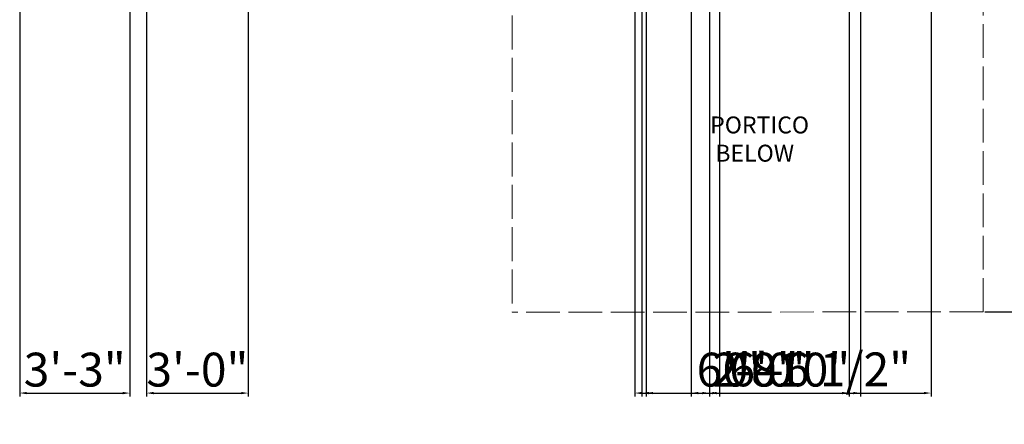
# Model space of a CAD drawing. Units: millimetres. Extents: x 542930 to 543750, y 628093 to 628738.
# Tile 1 of 14: x 542984 to 543333, y 628094 to 628237. Entities that reach past the tile are written whole.
import ezdxf

# ---------------------------------------------------------------- set-up
doc = ezdxf.new("R2010")
doc.units = ezdxf.units.MM
doc.linetypes.add('ACAD_ISO02W100', pattern=[15, 12, -3])
doc.layers.add('A-ANNO-DIMS', color=2, linetype='Continuous', lineweight=18)
doc.layers.add('A-FLOR-BELO', color=4, linetype='ACAD_ISO02W100', lineweight=18)
doc.layers.add('A-AREA-IDEN', color=40, linetype='Continuous', lineweight=18, true_color=0xf8d731)
doc.styles.get("Standard").update_dxf_attribs({"font": 'arial.ttf'})
doc.dimstyles.new('ISO-25', dxfattribs={"dimtxt": 12, "dimasz": 2.5, "dimexe": 1.25, "dimexo": 0.625, "dimtad": 1, "dimdec": 0, "dimlunit": 3, "dimtxsty": 'Standard', "dimcen": 2.5, "dimadec": 0, "dimazin": 0, "dimtfac": 1, "dimtdec": 0, "dimtmove": 0, "dimatfit": 3, "dimfxl": 1, "dimarcsym": 0})

# ---------------------------------------------------------------- blocks, each defined once
blk = doc.blocks.new('*D47')
at = {"layer": 'A-ANNO-DIMS', "color": 0, "lineweight": -2, "transparency": 16777216}
for p, q in [((542998.67, 628268.2), (542998.67, 628263.97)), ((543001.17, 628265.22), (543020.19, 628265.22)), ((543022.69, 628268.2), (543022.69, 628263.97)), ((543022.69, 628265.22), (543196.77, 628265.22))]:
    blk.add_line(p, q, dxfattribs=at)
at = {"layer": 'A-ANNO-DIMS', "color": 0, "transparency": 16777216}
for points in [[(543001.17, 628265.64), (543001.17, 628264.81), (542998.67, 628265.22)], [(543020.19, 628265.64), (543020.19, 628264.81), (543022.69, 628265.22)]]:
    blk.add_solid(points, dxfattribs=at)
at = {"layer": 'Defpoints', "color": 0, "transparency": 16777216}
for p in [(542998.67, 628268.83), (543022.69, 628268.83), (543022.69, 628265.22)]:
    blk.add_point(p, dxfattribs=at)
at = {"layer": 'A-ANNO-DIMS', "color": 0, "transparency": 16777216, "insert": (543110.98, 628271.97), "char_height": 12, "attachment_point": 5}
blk.add_mtext('END TABLE 2\'-0" TYP.', dxfattribs=at)
blk = doc.blocks.new('*D61')
at = {"layer": 'A-ANNO-DIMS', "color": 0, "lineweight": -2, "transparency": 16777216}
for p, q in [((543500.29, 628253.83), (543537.81, 628253.83)), ((543536.56, 628136.33), (543536.56, 628251.33)), ((543325.79, 628133.83), (543537.81, 628133.83))]:
    blk.add_line(p, q, dxfattribs=at)
at = {"layer": 'A-ANNO-DIMS', "color": 0, "transparency": 16777216}
for points in [[(543536.15, 628251.33), (543536.98, 628251.33), (543536.56, 628253.83)], [(543536.15, 628136.33), (543536.98, 628136.33), (543536.56, 628133.83)]]:
    blk.add_solid(points, dxfattribs=at)
at = {"layer": 'Defpoints', "color": 0, "transparency": 16777216}
for p in [(543499.67, 628253.83), (543536.56, 628253.83), (543325.17, 628133.83)]:
    blk.add_point(p, dxfattribs=at)
at = {"layer": 'A-ANNO-DIMS', "color": 0, "transparency": 16777216, "insert": (543529.81, 628193.83), "char_height": 12, "attachment_point": 5, "rotation": 90}
blk.add_mtext('10\'-0"', dxfattribs=at)
blk = doc.blocks.new('*D62')
at = {"layer": 'A-ANNO-DIMS', "color": 0, "lineweight": -2, "transparency": 16777216}
for p, q in [((542983.67, 628253.2), (542983.67, 628103.84)), ((543022.69, 628253.2), (543022.69, 628103.84)), ((542986.17, 628105.09), (543020.19, 628105.09))]:
    blk.add_line(p, q, dxfattribs=at)
at = {"layer": 'A-ANNO-DIMS', "color": 0, "transparency": 16777216}
for points in [[(542986.17, 628105.5), (542986.17, 628104.67), (542983.67, 628105.09)], [(543020.19, 628105.5), (543020.19, 628104.67), (543022.69, 628105.09)]]:
    blk.add_solid(points, dxfattribs=at)
at = {"layer": 'Defpoints', "color": 0, "transparency": 16777216}
for p in [(542983.67, 628253.83), (543022.69, 628253.83), (543022.69, 628105.09)]:
    blk.add_point(p, dxfattribs=at)
at = {"layer": 'A-ANNO-DIMS', "color": 0, "transparency": 16777216, "insert": (543003.18, 628111.84), "char_height": 12, "attachment_point": 5}
blk.add_mtext('3\'-3"', dxfattribs=at)
blk = doc.blocks.new('*D71')
at = {"layer": 'A-ANNO-DIMS', "color": 0, "lineweight": -2, "transparency": 16777216}
for p, q in [((543201.67, 628544.2), (543201.67, 628103.84)), ((543281.67, 628544.2), (543281.67, 628103.84)), ((543204.17, 628105.09), (543279.17, 628105.09))]:
    blk.add_line(p, q, dxfattribs=at)
at = {"layer": 'A-ANNO-DIMS', "color": 0, "transparency": 16777216}
for points in [[(543204.17, 628105.5), (543204.17, 628104.67), (543201.67, 628105.09)], [(543279.17, 628105.5), (543279.17, 628104.67), (543281.67, 628105.09)]]:
    blk.add_solid(points, dxfattribs=at)
at = {"layer": 'Defpoints', "color": 0, "transparency": 16777216}
for p in [(543201.67, 628544.83), (543281.67, 628544.83), (543281.67, 628105.09)]:
    blk.add_point(p, dxfattribs=at)
at = {"layer": 'A-ANNO-DIMS', "color": 0, "transparency": 16777216, "insert": (543241.67, 628111.84), "char_height": 12, "attachment_point": 5}
blk.add_mtext('6\'-8"', dxfattribs=at)
blk = doc.blocks.new('*D76')
at = {"layer": 'A-ANNO-DIMS', "color": 0, "lineweight": -2, "transparency": 16777216}
for p, q in [((543205.67, 628349.2), (543205.67, 628103.84)), ((543277.67, 628349.2), (543277.67, 628103.84)), ((543208.17, 628105.09), (543275.17, 628105.09))]:
    blk.add_line(p, q, dxfattribs=at)
at = {"layer": 'A-ANNO-DIMS', "color": 0, "transparency": 16777216}
for points in [[(543208.17, 628105.5), (543208.17, 628104.67), (543205.67, 628105.09)], [(543275.17, 628105.5), (543275.17, 628104.67), (543277.67, 628105.09)]]:
    blk.add_solid(points, dxfattribs=at)
at = {"layer": 'Defpoints', "color": 0, "transparency": 16777216}
for p in [(543205.67, 628349.83), (543277.67, 628349.83), (543277.67, 628105.09)]:
    blk.add_point(p, dxfattribs=at)
at = {"layer": 'A-ANNO-DIMS', "color": 0, "transparency": 16777216, "insert": (543241.67, 628111.84), "char_height": 12, "attachment_point": 5}
blk.add_mtext('6\'-0"', dxfattribs=at)
blk = doc.blocks.new('*D79')
at = {"layer": 'A-ANNO-DIMS', "color": 0, "lineweight": -2, "transparency": 16777216}
for p, q in [((543204.19, 628433.96), (543204.19, 628103.84)), ((543228.16, 628433.96), (543228.16, 628103.84)), ((543206.69, 628105.09), (543225.66, 628105.09)), ((543228.16, 628105.09), (543264.02, 628105.09))]:
    blk.add_line(p, q, dxfattribs=at)
at = {"layer": 'A-ANNO-DIMS', "color": 0, "transparency": 16777216}
for points in [[(543206.69, 628105.5), (543206.69, 628104.67), (543204.19, 628105.09)], [(543225.66, 628105.5), (543225.66, 628104.67), (543228.16, 628105.09)]]:
    blk.add_solid(points, dxfattribs=at)
at = {"layer": 'Defpoints', "color": 0, "transparency": 16777216}
for p in [(543204.19, 628434.59), (543228.16, 628434.59), (543228.16, 628105.09)]:
    blk.add_point(p, dxfattribs=at)
at = {"layer": 'A-ANNO-DIMS', "color": 0, "transparency": 16777216, "insert": (543247.34, 628111.84), "char_height": 12, "attachment_point": 5}
blk.add_mtext('2\'-0"', dxfattribs=at)
blk = doc.blocks.new('*D81')
at = {"layer": 'A-ANNO-DIMS', "color": 0, "lineweight": -2, "transparency": 16777216}
for p, q in [((543228.16, 628433.96), (543228.16, 628103.84)), ((543306.67, 628434.2), (543306.67, 628103.84)), ((543230.66, 628105.09), (543304.17, 628105.09))]:
    blk.add_line(p, q, dxfattribs=at)
at = {"layer": 'A-ANNO-DIMS', "color": 0, "transparency": 16777216}
for points in [[(543230.66, 628105.5), (543230.66, 628104.67), (543228.16, 628105.09)], [(543304.17, 628105.5), (543304.17, 628104.67), (543306.67, 628105.09)]]:
    blk.add_solid(points, dxfattribs=at)
at = {"layer": 'Defpoints', "color": 0, "transparency": 16777216}
for p in [(543228.16, 628434.59), (543306.67, 628434.83), (543306.67, 628105.09)]:
    blk.add_point(p, dxfattribs=at)
at = {"layer": 'A-ANNO-DIMS', "color": 0, "transparency": 16777216, "insert": (543267.41, 628111.92), "char_height": 12, "attachment_point": 5}
blk.add_mtext('6\'-6 1/2"', dxfattribs=at)
blk = doc.blocks.new('*D85')
at = {"layer": 'A-ANNO-DIMS', "color": 0, "lineweight": -2, "transparency": 16777216}
for p, q in [((543028.62, 628481.2), (543028.62, 628103.84)), ((543064.67, 628481.2), (543064.67, 628103.84)), ((543031.12, 628105.09), (543062.17, 628105.09))]:
    blk.add_line(p, q, dxfattribs=at)
at = {"layer": 'A-ANNO-DIMS', "color": 0, "transparency": 16777216}
for points in [[(543031.12, 628105.5), (543031.12, 628104.67), (543028.62, 628105.09)], [(543062.17, 628105.5), (543062.17, 628104.67), (543064.67, 628105.09)]]:
    blk.add_solid(points, dxfattribs=at)
at = {"layer": 'Defpoints', "color": 0, "transparency": 16777216}
for p in [(543028.62, 628481.83), (543064.67, 628481.83), (543064.67, 628105.09)]:
    blk.add_point(p, dxfattribs=at)
at = {"layer": 'A-ANNO-DIMS', "color": 0, "transparency": 16777216, "insert": (543046.65, 628111.84), "char_height": 12, "attachment_point": 5}
blk.add_mtext('3\'-0"', dxfattribs=at)
blk = doc.blocks.new('*D87')
at = {"layer": 'A-ANNO-DIMS', "color": 0, "lineweight": -2, "transparency": 16777216}
for p, q in [((543221.67, 628580.2), (543221.67, 628103.84)), ((543231.67, 628580.2), (543231.67, 628103.84)), ((543224.17, 628105.09), (543229.17, 628105.09)), ((543231.67, 628105.09), (543276.64, 628105.09))]:
    blk.add_line(p, q, dxfattribs=at)
at = {"layer": 'A-ANNO-DIMS', "color": 0, "transparency": 16777216}
for points in [[(543224.17, 628105.5), (543224.17, 628104.67), (543221.67, 628105.09)], [(543229.17, 628105.5), (543229.17, 628104.67), (543231.67, 628105.09)]]:
    blk.add_solid(points, dxfattribs=at)
at = {"layer": 'Defpoints', "color": 0, "transparency": 16777216}
for p in [(543221.67, 628580.83), (543231.67, 628580.83), (543231.67, 628105.09)]:
    blk.add_point(p, dxfattribs=at)
at = {"layer": 'A-ANNO-DIMS', "color": 0, "transparency": 16777216, "insert": (543255.4, 628111.84), "char_height": 12, "attachment_point": 5}
blk.add_mtext('0\'-10"', dxfattribs=at)

msp = doc.modelspace()

# ---------------------------------------------------------------- linework, layer by layer
at = {"layer": 'A-FLOR-BELO'}
for p, q in [((543325.17, 628340.83), (543325.17, 628133.83)), ((543158.17, 628253.83), (543158.17, 628133.79)), ((543325.17, 628133.83), (543158.17, 628133.79))]:
    msp.add_line(p, q, dxfattribs=at)

# ---------------------------------------------------------------- texts
at = {"layer": 'A-AREA-IDEN', "insert": (543222.89, 628203.09), "char_height": 6, "attachment_point": 1}
msp.add_mtext_dynamic_manual_height_columns('   PORTICO\\P    BELOW', width=77.2525, gutter_width=12.5, heights=[0], dxfattribs=at)

# ---------------------------------------------------------------- dimensions: what is measured, and where the dimension line sits
at = {"layer": 'A-ANNO-DIMS'}
for base, p1, p2, picture, middle in [((543231.67, 628105.09), (543221.67, 628580.83), (543231.67, 628580.83), '*D87', (543255.4, 628111.84)), ((543281.67, 628105.09), (543201.67, 628544.83), (543281.67, 628544.83), '*D71', (543241.67, 628111.84)), ((543064.6669, 628105.0858), (543028.6237, 628481.8258), (543064.6669, 628481.8258), '*D85', (543046.6453, 628111.8418)), ((543228.16, 628105.09), (543204.19, 628434.59), (543228.16, 628434.59), '*D79', (543247.34, 628111.84)), ((543306.67, 628105.09), (543228.16, 628434.59), (543306.67, 628434.83), '*D81', (543267.41, 628111.92)), ((543277.67, 628105.09), (543205.67, 628349.83), (543277.67, 628349.83), '*D76', (543241.67, 628111.84)), ((543022.69, 628105.09), (542983.67, 628253.83), (543022.69, 628253.83), '*D62', (543003.18, 628111.84))]:
    dim = msp.add_linear_dim(base=base, p1=p1, p2=p2, dimstyle='ISO-25', override={"dimdec": 1, "dimlfac": 1, "dimrnd": 0, "dimzin": 1, "dimdsep": 46, "dimlunit": 4, "dimfrac": 2}, dxfattribs=at)
    dim.commit()
    dim.dimension.update_dxf_attribs({"geometry": picture, "text_midpoint": middle})
dim = msp.add_linear_dim(base=(543022.69, 628265.22), p1=(542998.67, 628268.83), p2=(543022.69, 628268.83), text='END TABLE <> TYP.', dimstyle='ISO-25', override={"dimdec": 1, "dimlfac": 1, "dimrnd": 0, "dimzin": 1, "dimdsep": 46, "dimlunit": 4, "dimfrac": 2}, dxfattribs=at)
dim.commit()
dim.dimension.update_dxf_attribs({"geometry": '*D47', "text_midpoint": (543110.98, 628271.97)})
dim = msp.add_linear_dim(base=(543536.56, 628253.83), p1=(543325.17, 628133.83), p2=(543499.67, 628253.83), angle=90, dimstyle='ISO-25', override={"dimdec": 1, "dimlfac": 1, "dimrnd": 0, "dimzin": 1, "dimdsep": 46, "dimlunit": 4, "dimfrac": 2}, dxfattribs=at)
dim.commit()
dim.dimension.update_dxf_attribs({"geometry": '*D61', "text_midpoint": (543529.81, 628193.83)})

doc.saveas('drawing.dxf')
